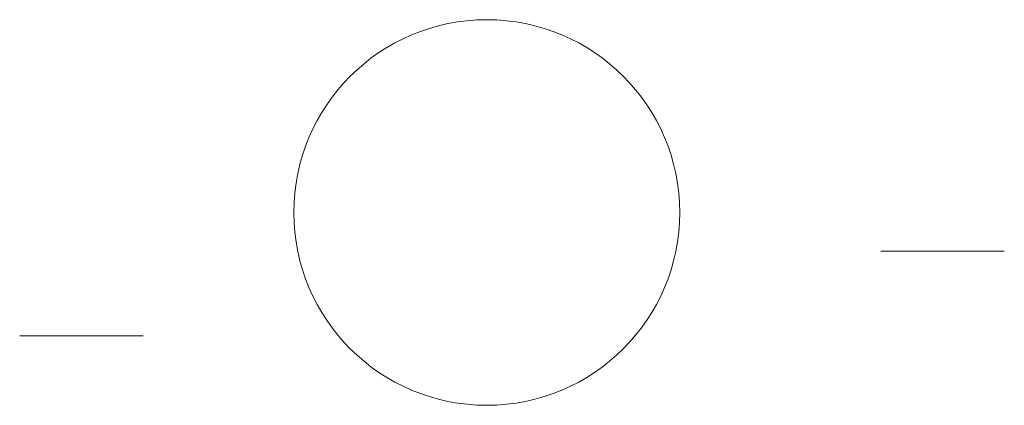
# Model space of a CAD drawing. Units: millimetres. Extents: x -61 to 67, y -25 to 25.
import ezdxf

# ---------------------------------------------------------------- set-up
doc = ezdxf.new("R2010")
doc.units = ezdxf.units.MM
doc.layers.add('M-CONS', color=9, linetype='Continuous', lineweight=13)

msp = doc.modelspace()

# ---------------------------------------------------------------- linework, layer by layer
at = {"layer": 'M-CONS'}
msp.add_circle((0, 0), 25, dxfattribs=at)
at = {"layer": 'M-CONS', "extrusion": (0, 1, 0)}
for centre in [(-59.05, 26.47, -5), (52.51, 28, -16)]:
    msp.add_circle(centre, 8, dxfattribs=at)

doc.saveas('drawing.dxf')
